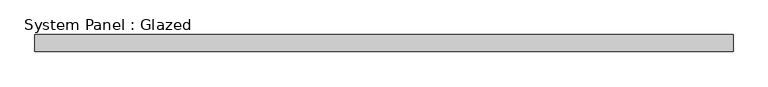
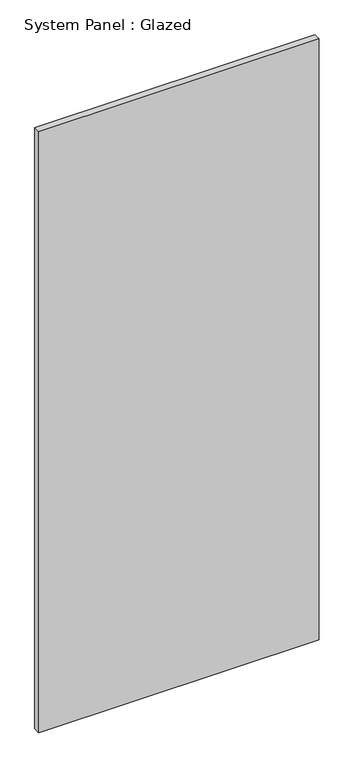
"""IFC4 building model written with IfcOpenShell, lengths in millimetres: plate geometry, System Panel : Glazed."""

from ifc_helpers import new_model, si_unit, origin, origin_with_axes, place, context, project, spatial, polyline, outline, extrude, source, transform, mapped, element, save


def system_panel_glazed_66ef8e2c(model_context):
    return source(origin(), model_context, "Body", "SweptSolid", [
        extrude(outline(polyline([(523.875, 19.05), (-523.875, 19.05), (-523.875, 44.45), (523.875, 44.45), (523.875, 19.05)])), origin_with_axes(), (0.0, 0.0, 1.0), 2374.9),
    ])


if __name__ == "__main__":
    model = new_model("IFC4")
    model_context = context("Model", 3, world=origin())
    ifc_project = project(units=[si_unit("LENGTHUNIT", "METRE", prefix="MILLI")], contexts=[model_context])
    site = spatial("IfcSite", under=ifc_project)
    building = spatial("IfcBuilding", under=site)
    placement = place(None, origin())
    system_panel_glazed_shape = system_panel_glazed_66ef8e2c(model_context)
    element("IfcPlate", 1, ObjectType="System Panel : Glazed", at=placement, inside=building, context=model_context, shape_type="MappedRepresentation", body=[
        mapped(system_panel_glazed_shape, transform((0.0, 0.0, 0.0), x_axis=(1.0, 0.0, 0.0), y_axis=(0.0, 1.0, 0.0), z_axis=(0.0, 0.0, 1.0))),
    ])
    save(model, "model.ifc")

# Revit data of these elements
# Type "System Panel : Glazed"
#   Construction Type Id = "GSP4R"
#   Analytic Construction = "1/8 in Pilkington single glazing"
#   Visual Light Transmittance = 0.9
#   Solar Heat Gain Coefficient = 0.86
#   Heat Transfer Coefficient (U) = 1.18115 BTU/(h·ft²·°F)
#   Define Thermal Properties by = 1
# Element 1 (IfcPlate, "System Panel : Glazed")
#   Materials on its faces: "Glass"
# Materials
#   "Glass": class "Glass", colour RGB 0 128 192, transparency 0.75, Description = "Soda Lime Glass", Cost = 0
